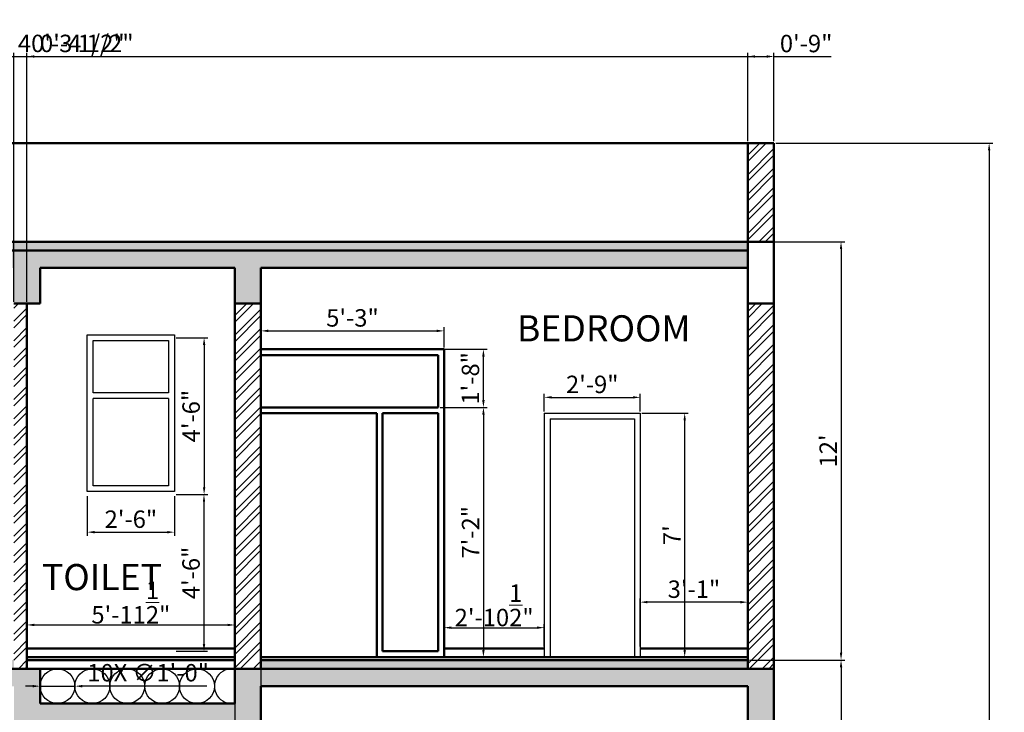
# Model space of a CAD drawing. Units: inches. Extents: x 1615 to 2231, y 1931 to 2519.
# Tile 6 of 6: x 1892 to 2231, y 2281 to 2519. Entities that reach past the tile are written whole.
import ezdxf

# ---------------------------------------------------------------- set-up
doc = ezdxf.new("R2010")
doc.units = ezdxf.units.IN
for name, color, linetype, lineweight in [('A-ANNO-DIMS', 2, 'Continuous', 18), ('A-AREA-IDEN', 7, 'Continuous', 25), ('A-DOOR', 3, 'Continuous', 25), ('A-GLAZ', 4, 'Continuous', 25), ('A-SECT', 7, 'Continuous', 50), ('A-WALL-PATT', 8, 'Continuous', 13), ('S-SLAB', 7, 'Continuous', 25)]:
    doc.layers.add(name, color=color, linetype=linetype, lineweight=lineweight)
doc.styles.get("Standard").update_dxf_attribs({"font": 'arial.ttf'})
doc.dimstyles.new('ISO-25', dxfattribs={"dimtxt": 6, "dimasz": 2.5, "dimexe": 1.25, "dimexo": 0.625, "dimtad": 1, "dimdec": 1, "dimlunit": 4, "dimtxsty": 'Standard', "dimcen": 2.5, "dimadec": 0, "dimazin": 0, "dimtfac": 1, "dimtdec": 1, "dimtmove": 0, "dimatfit": 3, "dimfxl": 1, "dimarcsym": 0})

# ---------------------------------------------------------------- blocks, each defined once
blk = doc.blocks.new('*D37')
at = {"layer": 'A-ANNO-DIMS', "color": 0, "lineweight": -2, "transparency": 16777216}
for p, q in [((1915.12, 2354.9), (1915.12, 2341.31)), ((1945.12, 2354.9), (1945.12, 2341.31)), ((1917.62, 2342.56), (1942.62, 2342.56))]:
    blk.add_line(p, q, dxfattribs=at)
at = {"layer": 'A-ANNO-DIMS', "color": 0, "lineweight": 100, "transparency": 16777216}
for points in [[(1917.62, 2342.98), (1917.62, 2342.14), (1915.12, 2342.56)], [(1942.62, 2342.98), (1942.62, 2342.14), (1945.12, 2342.56)]]:
    blk.add_solid(points, dxfattribs=at)
at = {"layer": 'Defpoints', "color": 0, "lineweight": 100, "transparency": 16777216}
for p in [(1915.12, 2355.53), (1945.12, 2355.53), (1945.12, 2342.56)]:
    blk.add_point(p, dxfattribs=at)
at = {"layer": 'A-ANNO-DIMS', "color": 0, "transparency": 16777216, "insert": (1930.12, 2346.25), "char_height": 6, "attachment_point": 5}
blk.add_mtext('2\'-6"', dxfattribs=at)
blk = doc.blocks.new('*D38')
at = {"layer": 'A-ANNO-DIMS', "color": 0, "lineweight": -2, "transparency": 16777216}
for p, q in [((1945.74, 2409.53), (1956.57, 2409.53)), ((1955.32, 2407.03), (1955.32, 2358.03)), ((1945.74, 2355.53), (1956.57, 2355.53))]:
    blk.add_line(p, q, dxfattribs=at)
at = {"layer": 'A-ANNO-DIMS', "color": 0, "lineweight": 100, "transparency": 16777216}
for points in [[(1954.91, 2407.03), (1955.74, 2407.03), (1955.32, 2409.53)], [(1954.91, 2358.03), (1955.74, 2358.03), (1955.32, 2355.53)]]:
    blk.add_solid(points, dxfattribs=at)
at = {"layer": 'Defpoints', "color": 0, "lineweight": 100, "transparency": 16777216}
for p in [(1945.12, 2409.53), (1945.12, 2355.53), (1955.32, 2355.53)]:
    blk.add_point(p, dxfattribs=at)
at = {"layer": 'A-ANNO-DIMS', "color": 0, "transparency": 16777216, "insert": (1951.63, 2382.53), "char_height": 6, "attachment_point": 5, "rotation": 90}
blk.add_mtext('4\'-6"', dxfattribs=at)
blk = doc.blocks.new('*D39')
at = {"layer": 'A-ANNO-DIMS', "color": 0, "lineweight": -2, "transparency": 16777216}
for p, q in [((1945.74, 2355.53), (1956.53, 2355.53)), ((1955.28, 2353.03), (1955.28, 2304.03)), ((1945.74, 2301.53), (1956.53, 2301.53))]:
    blk.add_line(p, q, dxfattribs=at)
at = {"layer": 'A-ANNO-DIMS', "color": 0, "lineweight": 100, "transparency": 16777216}
for points in [[(1954.87, 2353.03), (1955.7, 2353.03), (1955.28, 2355.53)], [(1954.87, 2304.03), (1955.7, 2304.03), (1955.28, 2301.53)]]:
    blk.add_solid(points, dxfattribs=at)
at = {"layer": 'Defpoints', "color": 0, "lineweight": 100, "transparency": 16777216}
for p in [(1945.12, 2355.53), (1945.12, 2301.53), (1955.28, 2301.53)]:
    blk.add_point(p, dxfattribs=at)
at = {"layer": 'A-ANNO-DIMS', "color": 0, "transparency": 16777216, "insert": (1951.6, 2328.53), "char_height": 6, "attachment_point": 5, "rotation": 90}
blk.add_mtext('4\'-6"', dxfattribs=at)
blk = doc.blocks.new('*D46')
at = {"layer": 'A-ANNO-DIMS', "color": 0, "lineweight": -2, "transparency": 16777216}
for p, q in [((2037.87, 2303.15), (2037.87, 2310.92)), ((2072.37, 2303.15), (2072.37, 2310.92)), ((2040.37, 2309.67), (2069.87, 2309.67))]:
    blk.add_line(p, q, dxfattribs=at)
at = {"layer": 'A-ANNO-DIMS', "color": 0, "lineweight": 100, "transparency": 16777216}
for points in [[(2040.37, 2310.09), (2040.37, 2309.25), (2037.87, 2309.67)], [(2069.87, 2310.09), (2069.87, 2309.25), (2072.37, 2309.67)]]:
    blk.add_solid(points, dxfattribs=at)
at = {"layer": 'Defpoints', "color": 0, "lineweight": 100, "transparency": 16777216}
for p in [(2072.37, 2309.67), (2037.87, 2302.53), (2072.37, 2302.53)]:
    blk.add_point(p, dxfattribs=at)
at = {"layer": 'A-ANNO-DIMS', "color": 0, "transparency": 16777216, "insert": (2055.12, 2317.37), "char_height": 6, "attachment_point": 5}
blk.add_mtext('2\'-10{\\H1x;\\S1/2;}"', dxfattribs=at)
blk = doc.blocks.new('*D47')
at = {"layer": 'A-ANNO-DIMS', "color": 0, "lineweight": -2, "transparency": 16777216}
for p, q in [((2105.99, 2383.53), (2121.93, 2383.53)), ((2120.68, 2302.03), (2120.68, 2381.03)), ((2105.99, 2299.53), (2121.93, 2299.53))]:
    blk.add_line(p, q, dxfattribs=at)
at = {"layer": 'A-ANNO-DIMS', "color": 0, "lineweight": 100, "transparency": 16777216}
for points in [[(2120.27, 2381.03), (2121.1, 2381.03), (2120.68, 2383.53)], [(2120.27, 2302.03), (2121.1, 2302.03), (2120.68, 2299.53)]]:
    blk.add_solid(points, dxfattribs=at)
at = {"layer": 'Defpoints', "color": 0, "lineweight": 100, "transparency": 16777216}
for p in [(2105.37, 2383.53), (2120.68, 2383.53), (2105.37, 2299.53)]:
    blk.add_point(p, dxfattribs=at)
at = {"layer": 'A-ANNO-DIMS', "color": 0, "transparency": 16777216, "insert": (2117.06, 2341.53), "char_height": 6, "attachment_point": 5, "rotation": 90}
blk.add_mtext("7'", dxfattribs=at)
blk = doc.blocks.new('*D48')
at = {"layer": 'A-ANNO-DIMS', "color": 0, "lineweight": -2, "transparency": 16777216}
for p, q in [((2072.37, 2384.15), (2072.37, 2390.23)), ((2074.87, 2388.98), (2102.87, 2388.98)), ((2105.37, 2384.15), (2105.37, 2390.23))]:
    blk.add_line(p, q, dxfattribs=at)
at = {"layer": 'A-ANNO-DIMS', "color": 0, "lineweight": 100, "transparency": 16777216}
for points in [[(2074.87, 2389.4), (2074.87, 2388.57), (2072.37, 2388.98)], [(2102.87, 2389.4), (2102.87, 2388.57), (2105.37, 2388.98)]]:
    blk.add_solid(points, dxfattribs=at)
at = {"layer": 'Defpoints', "color": 0, "lineweight": 100, "transparency": 16777216}
for p in [(2105.37, 2388.98), (2072.37, 2383.53), (2105.37, 2383.53)]:
    blk.add_point(p, dxfattribs=at)
at = {"layer": 'A-ANNO-DIMS', "color": 0, "transparency": 16777216, "insert": (2088.87, 2392.67), "char_height": 6, "attachment_point": 5}
blk.add_mtext('2\'-9"', dxfattribs=at)
blk = doc.blocks.new('*D54')
at = {"layer": 'A-ANNO-DIMS', "color": 0, "lineweight": -2, "transparency": 16777216}
for p, q in [((2036.49, 2405.53), (2052.68, 2405.53)), ((2051.43, 2388.03), (2051.43, 2403.03)), ((2036.49, 2385.53), (2052.68, 2385.53))]:
    blk.add_line(p, q, dxfattribs=at)
at = {"layer": 'A-ANNO-DIMS', "color": 0, "lineweight": 100, "transparency": 16777216}
for points in [[(2051.01, 2403.03), (2051.85, 2403.03), (2051.43, 2405.53)], [(2051.01, 2388.03), (2051.85, 2388.03), (2051.43, 2385.53)]]:
    blk.add_solid(points, dxfattribs=at)
at = {"layer": 'Defpoints', "color": 0, "lineweight": 100, "transparency": 16777216}
for p in [(2035.87, 2405.53), (2051.43, 2405.53), (2035.87, 2385.53)]:
    blk.add_point(p, dxfattribs=at)
at = {"layer": 'A-ANNO-DIMS', "color": 0, "transparency": 16777216, "insert": (2047.74, 2395.53), "char_height": 6, "attachment_point": 5, "rotation": 90}
blk.add_mtext('1\'-8"', dxfattribs=at)
blk = doc.blocks.new('*D55')
at = {"layer": 'A-ANNO-DIMS', "color": 0, "lineweight": -2, "transparency": 16777216}
for p, q in [((2036.49, 2385.53), (2052.68, 2385.53)), ((2051.43, 2383.03), (2051.43, 2302.03)), ((2036.49, 2299.53), (2052.68, 2299.53))]:
    blk.add_line(p, q, dxfattribs=at)
at = {"layer": 'A-ANNO-DIMS', "color": 0, "lineweight": 100, "transparency": 16777216}
for points in [[(2051.01, 2383.03), (2051.85, 2383.03), (2051.43, 2385.53)], [(2051.01, 2302.03), (2051.85, 2302.03), (2051.43, 2299.53)]]:
    blk.add_solid(points, dxfattribs=at)
at = {"layer": 'Defpoints', "color": 0, "lineweight": 100, "transparency": 16777216}
for p in [(2035.87, 2385.53), (2035.87, 2299.53), (2051.43, 2299.53)]:
    blk.add_point(p, dxfattribs=at)
at = {"layer": 'A-ANNO-DIMS', "color": 0, "transparency": 16777216, "insert": (2047.79, 2342.53), "char_height": 6, "attachment_point": 5, "rotation": 90}
blk.add_mtext('7\'-2"', dxfattribs=at)
blk = doc.blocks.new('*D56')
at = {"layer": 'A-ANNO-DIMS', "color": 0, "lineweight": -2, "transparency": 16777216}
for p, q in [((1974.87, 2406.15), (1974.87, 2413.12)), ((2037.87, 2406.15), (2037.87, 2413.12)), ((1977.37, 2411.87), (2035.37, 2411.87))]:
    blk.add_line(p, q, dxfattribs=at)
at = {"layer": 'A-ANNO-DIMS', "color": 0, "lineweight": 100, "transparency": 16777216}
for points in [[(1977.37, 2412.29), (1977.37, 2411.46), (1974.87, 2411.87)], [(2035.37, 2412.29), (2035.37, 2411.46), (2037.87, 2411.87)]]:
    blk.add_solid(points, dxfattribs=at)
at = {"layer": 'Defpoints', "color": 0, "lineweight": 100, "transparency": 16777216}
for p in [(2037.87, 2411.87), (1974.87, 2405.53), (2037.87, 2405.53)]:
    blk.add_point(p, dxfattribs=at)
at = {"layer": 'A-ANNO-DIMS', "color": 0, "transparency": 16777216, "insert": (2006.37, 2415.56), "char_height": 6, "attachment_point": 5}
blk.add_mtext('5\'-3"', dxfattribs=at)
blk = doc.blocks.new('*D57')
at = {"layer": 'A-ANNO-DIMS', "color": 0, "lineweight": -2, "transparency": 16777216}
for p, q in [((2105.37, 2303.15), (2105.37, 2319.71)), ((2139.87, 2318.46), (2107.87, 2318.46)), ((2142.37, 2303.15), (2142.37, 2319.71))]:
    blk.add_line(p, q, dxfattribs=at)
at = {"layer": 'A-ANNO-DIMS', "color": 0, "lineweight": 100, "transparency": 16777216}
for points in [[(2107.87, 2318.88), (2107.87, 2318.05), (2105.37, 2318.46)], [(2139.87, 2318.88), (2139.87, 2318.05), (2142.37, 2318.46)]]:
    blk.add_solid(points, dxfattribs=at)
at = {"layer": 'Defpoints', "color": 0, "lineweight": 100, "transparency": 16777216}
for p in [(2105.37, 2318.46), (2105.37, 2302.53), (2142.37, 2302.53)]:
    blk.add_point(p, dxfattribs=at)
at = {"layer": 'A-ANNO-DIMS', "color": 0, "transparency": 16777216, "insert": (2123.87, 2322.15), "char_height": 6, "attachment_point": 5}
blk.add_mtext('3\'-1"', dxfattribs=at)
blk = doc.blocks.new('*D61')
at = {"layer": 'A-ANNO-DIMS', "color": 0, "lineweight": -2, "transparency": 16777216}
for p, q in [((1894.37, 2303.15), (1894.37, 2311.86)), ((1896.87, 2310.61), (1963.37, 2310.61)), ((1965.87, 2303.15), (1965.87, 2311.86))]:
    blk.add_line(p, q, dxfattribs=at)
at = {"layer": 'A-ANNO-DIMS', "color": 0, "lineweight": 100, "transparency": 16777216}
for points in [[(1896.87, 2311.03), (1896.87, 2310.19), (1894.37, 2310.61)], [(1963.37, 2311.03), (1963.37, 2310.19), (1965.87, 2310.61)]]:
    blk.add_solid(points, dxfattribs=at)
at = {"layer": 'Defpoints', "color": 0, "lineweight": 100, "transparency": 16777216}
for p in [(1965.87, 2310.61), (1894.37, 2302.53), (1965.87, 2302.53)]:
    blk.add_point(p, dxfattribs=at)
at = {"layer": 'A-ANNO-DIMS', "color": 0, "transparency": 16777216, "insert": (1930.12, 2318.31), "char_height": 6, "attachment_point": 5}
blk.add_mtext('5\'-11{\\H1x;\\S1/2;}"', dxfattribs=at)
blk = doc.blocks.new('*D62')
at = {"layer": 'A-ANNO-DIMS', "color": 0, "lineweight": -2, "transparency": 16777216}
for p, q in [((2142.99, 2442.53), (2175.73, 2442.53)), ((2174.48, 2440.03), (2174.48, 2301.03)), ((2142.99, 2298.53), (2175.73, 2298.53))]:
    blk.add_line(p, q, dxfattribs=at)
at = {"layer": 'A-ANNO-DIMS', "color": 0, "lineweight": 100, "transparency": 16777216}
for points in [[(2174.07, 2440.03), (2174.9, 2440.03), (2174.48, 2442.53)], [(2174.07, 2301.03), (2174.9, 2301.03), (2174.48, 2298.53)]]:
    blk.add_solid(points, dxfattribs=at)
at = {"layer": 'Defpoints', "color": 0, "lineweight": 100, "transparency": 16777216}
for p in [(2142.37, 2442.53), (2142.37, 2298.53), (2174.48, 2298.53)]:
    blk.add_point(p, dxfattribs=at)
at = {"layer": 'A-ANNO-DIMS', "color": 0, "transparency": 16777216, "insert": (2170.85, 2370.53), "char_height": 6, "attachment_point": 5, "rotation": 90}
blk.add_mtext("12'", dxfattribs=at)
blk = doc.blocks.new('*D63')
at = {"layer": 'A-ANNO-DIMS', "color": 0, "lineweight": -2, "transparency": 16777216}
for p, q in [((2142.99, 2298.53), (2175.73, 2298.53)), ((2174.48, 2296.03), (2174.48, 2157.03)), ((2142.99, 2154.53), (2175.73, 2154.53))]:
    blk.add_line(p, q, dxfattribs=at)
at = {"layer": 'A-ANNO-DIMS', "color": 0, "lineweight": 100, "transparency": 16777216}
for points in [[(2174.07, 2296.03), (2174.9, 2296.03), (2174.48, 2298.53)], [(2174.07, 2157.03), (2174.9, 2157.03), (2174.48, 2154.53)]]:
    blk.add_solid(points, dxfattribs=at)
at = {"layer": 'Defpoints', "color": 0, "lineweight": 100, "transparency": 16777216}
for p in [(2142.37, 2298.53), (2142.37, 2154.53), (2174.48, 2154.53)]:
    blk.add_point(p, dxfattribs=at)
at = {"layer": 'A-ANNO-DIMS', "color": 0, "transparency": 16777216, "insert": (2170.85, 2226.53), "char_height": 6, "attachment_point": 5, "rotation": 90}
blk.add_mtext("12'", dxfattribs=at)
blk = doc.blocks.new('WIN-TOILET')
for p, q in [((1915.12, 2410.53), (1945.12, 2410.53)), ((1915.12, 2356.53), (1915.12, 2410.53)), ((1945.12, 2410.53), (1945.12, 2390.53)), ((1917.12, 2408.53), (1943.12, 2408.53)), ((1917.12, 2390.53), (1917.12, 2408.53)), ((1943.12, 2408.53), (1943.12, 2390.53)), ((1943.12, 2390.53), (1917.12, 2390.53)), ((1943.12, 2388.53), (1917.12, 2388.53)), ((1917.12, 2358.53), (1917.12, 2388.53)), ((1943.12, 2388.53), (1943.12, 2358.53)), ((1945.12, 2390.53), (1945.12, 2356.53)), ((1943.12, 2358.53), (1917.12, 2358.53)), ((1945.12, 2356.53), (1915.12, 2356.53))]:
    blk.add_line(p, q)
blk = doc.blocks.new('DOOR-KITCHEN')
for p, q in [((2072.37, 2383.53), (2072.37, 2299.53)), ((2072.37, 2383.53), (2105.37, 2383.53)), ((2105.37, 2383.53), (2105.37, 2299.53)), ((2074.37, 2381.53), (2103.37, 2381.53)), ((2074.37, 2381.53), (2074.37, 2299.53)), ((2103.37, 2381.53), (2103.37, 2299.53))]:
    blk.add_line(p, q)
blk = doc.blocks.new('*D78')
at = {"layer": 'A-ANNO-DIMS', "color": 0, "lineweight": -2, "transparency": 16777216}
for p, q in [((1667.87, 2477.15), (1667.87, 2507.6)), ((2151.37, 2477.15), (2151.37, 2507.6)), ((1670.37, 2506.35), (2148.87, 2506.35))]:
    blk.add_line(p, q, dxfattribs=at)
at = {"layer": 'A-ANNO-DIMS', "color": 0, "lineweight": 100, "transparency": 16777216}
for points in [[(1670.37, 2506.77), (1670.37, 2505.93), (1667.87, 2506.35)], [(2148.87, 2506.77), (2148.87, 2505.93), (2151.37, 2506.35)]]:
    blk.add_solid(points, dxfattribs=at)
at = {"layer": 'Defpoints', "color": 0, "lineweight": 100, "transparency": 16777216}
for p in [(2151.37, 2506.35), (1667.87, 2476.53), (2151.37, 2476.53)]:
    blk.add_point(p, dxfattribs=at)
at = {"layer": 'A-ANNO-DIMS', "color": 0, "transparency": 16777216, "insert": (1909.62, 2510.08), "char_height": 6, "attachment_point": 5}
blk.add_mtext('40\'-3 1/2"', dxfattribs=at)
blk = doc.blocks.new('*D79')
at = {"layer": 'A-ANNO-DIMS', "color": 0, "lineweight": -2, "transparency": 16777216}
for p, q in [((2151.99, 2476.53), (2226.69, 2476.53)), ((2225.44, 2474.03), (2225.44, 2004.53)), ((2175.99, 2002.03), (2226.69, 2002.03))]:
    blk.add_line(p, q, dxfattribs=at)
at = {"layer": 'A-ANNO-DIMS', "color": 0, "lineweight": 100, "transparency": 16777216}
for points in [[(2225.02, 2474.03), (2225.86, 2474.03), (2225.44, 2476.53)], [(2225.02, 2004.53), (2225.86, 2004.53), (2225.44, 2002.03)]]:
    blk.add_solid(points, dxfattribs=at)
at = {"layer": 'Defpoints', "color": 0, "lineweight": 100, "transparency": 16777216}
for p in [(2151.37, 2476.53), (2175.37, 2002.03), (2225.44, 2002.03)]:
    blk.add_point(p, dxfattribs=at)
at = {"layer": 'A-ANNO-DIMS', "color": 0, "transparency": 16777216, "insert": (2221.71, 2239.28), "char_height": 6, "attachment_point": 5, "rotation": 90}
blk.add_mtext('39\'-6 1/2"', dxfattribs=at)
blk = doc.blocks.new('*D81')
at = {"layer": 'A-ANNO-DIMS', "color": 0, "lineweight": -2, "transparency": 16777216}
for p, q in [((2142.37, 2477.15), (2142.37, 2507.6)), ((2151.37, 2477.15), (2151.37, 2507.6)), ((2144.87, 2506.35), (2148.87, 2506.35)), ((2151.37, 2506.35), (2171.07, 2506.35))]:
    blk.add_line(p, q, dxfattribs=at)
at = {"layer": 'A-ANNO-DIMS', "color": 0, "lineweight": 100, "transparency": 16777216}
for points in [[(2144.87, 2506.77), (2144.87, 2505.93), (2142.37, 2506.35)], [(2148.87, 2506.77), (2148.87, 2505.93), (2151.37, 2506.35)]]:
    blk.add_solid(points, dxfattribs=at)
at = {"layer": 'Defpoints', "color": 0, "lineweight": 100, "transparency": 16777216}
for p in [(2151.37, 2506.35), (2142.37, 2476.53), (2151.37, 2476.53)]:
    blk.add_point(p, dxfattribs=at)
at = {"layer": 'A-ANNO-DIMS', "color": 0, "transparency": 16777216, "insert": (2162.47, 2510.04), "char_height": 6, "attachment_point": 5}
blk.add_mtext('0\'-9"', dxfattribs=at)
blk = doc.blocks.new('*D82')
at = {"layer": 'A-ANNO-DIMS', "color": 0, "lineweight": -2, "transparency": 16777216}
for p, q in [((1889.87, 2421.92), (1889.87, 2507.6)), ((1894.37, 2421.92), (1894.37, 2507.6)), ((1887.37, 2506.35), (1884.87, 2506.35)), ((1889.87, 2506.35), (1894.37, 2506.35)), ((1896.87, 2506.35), (1930.55, 2506.35))]:
    blk.add_line(p, q, dxfattribs=at)
at = {"layer": 'A-ANNO-DIMS', "color": 0, "lineweight": 100, "transparency": 16777216}
for points in [[(1887.37, 2506.77), (1887.37, 2505.93), (1889.87, 2506.35)], [(1896.87, 2506.77), (1896.87, 2505.93), (1894.37, 2506.35)]]:
    blk.add_solid(points, dxfattribs=at)
at = {"layer": 'Defpoints', "color": 0, "lineweight": 100, "transparency": 16777216}
for p in [(1894.37, 2506.35), (1889.87, 2421.29), (1894.37, 2421.29)]:
    blk.add_point(p, dxfattribs=at)
at = {"layer": 'A-ANNO-DIMS', "color": 0, "transparency": 16777216, "insert": (1914.96, 2510.08), "char_height": 6, "attachment_point": 5}
blk.add_mtext('0\'-4 1/2"', dxfattribs=at)
blk = doc.blocks.new('*D83')
at = {"layer": 'A-ANNO-DIMS', "color": 0, "lineweight": -2, "transparency": 16777216}
for p, q in [((1965.87, 2420.67), (1965.87, 1970.95)), ((1974.87, 2420.67), (1974.87, 1970.95)), ((1968.37, 1972.2), (1972.37, 1972.2)), ((1974.87, 1972.2), (1994.57, 1972.2))]:
    blk.add_line(p, q, dxfattribs=at)
at = {"layer": 'A-ANNO-DIMS', "color": 0, "lineweight": 100, "transparency": 16777216}
for points in [[(1968.37, 1972.62), (1968.37, 1971.78), (1965.87, 1972.2)], [(1972.37, 1972.62), (1972.37, 1971.78), (1974.87, 1972.2)]]:
    blk.add_solid(points, dxfattribs=at)
at = {"layer": 'Defpoints', "color": 0, "lineweight": 100, "transparency": 16777216}
for p in [(1965.87, 2421.29), (1974.87, 2421.29), (1974.87, 1972.2)]:
    blk.add_point(p, dxfattribs=at)
at = {"layer": 'A-ANNO-DIMS', "color": 0, "transparency": 16777216, "insert": (1985.97, 1975.89), "char_height": 6, "attachment_point": 5}
blk.add_mtext('0\'-9"', dxfattribs=at)
blk = doc.blocks.new('*D91')
at = {"layer": 'A-ANNO-DIMS', "color": 0, "lineweight": -2, "transparency": 16777216}
for p, q in [((1896.37, 2289.53), (1893.87, 2289.53)), ((1898.87, 2289.53), (1910.87, 2289.53)), ((1956.26, 2289.53), (1913.37, 2289.53))]:
    blk.add_line(p, q, dxfattribs=at)
at = {"layer": 'A-ANNO-DIMS', "color": 0, "lineweight": 100, "transparency": 16777216}
for points in [[(1896.37, 2289.94), (1896.37, 2289.11), (1898.87, 2289.53)], [(1913.37, 2289.94), (1913.37, 2289.11), (1910.87, 2289.53)]]:
    blk.add_solid(points, dxfattribs=at)
at = {"layer": 'Defpoints', "color": 0, "lineweight": 100, "transparency": 16777216}
for p in [(1898.87, 2289.53), (1910.87, 2289.53)]:
    blk.add_point(p, dxfattribs=at)
at = {"layer": 'A-ANNO-DIMS', "color": 0, "transparency": 16777216, "insert": (1936.06, 2293.38), "char_height": 6, "attachment_point": 5, "rotation": 0.0032}
blk.add_mtext('10X ∅1\'-0"', dxfattribs=at)

msp = doc.modelspace()

# ---------------------------------------------------------------- hatches: boundary and pattern name
at = {"layer": 'A-WALL-PATT'}
h = msp.add_hatch(dxfattribs=at)
h.set_pattern_fill('ANSI32', color=256, scale=0.5)
h.paths.add_polyline_path([(1676.87, 2421.53), (1667.87, 2421.53), (1667.87, 2295.53), (1676.87, 2295.53)])
h.paths.add_polyline_path([(1676.87, 2277.53), (1667.87, 2277.53), (1667.87, 2151.53), (1676.87, 2151.53)])
h.paths.add_polyline_path([(1676.87, 2476.53), (1667.87, 2476.53), (1667.87, 2439.53), (1676.87, 2439.53)])
h.paths.add_polyline_path([(1894.37, 2421.29), (1889.87, 2421.29), (1889.87, 2295.53), (1894.37, 2295.53)])
h.paths.add_polyline_path([(1974.87, 2421.29), (1965.87, 2421.29), (1965.87, 2295.53), (1974.87, 2295.53)])
h.paths.add_polyline_path([(2151.37, 2421.29), (2142.37, 2421.29), (2142.37, 2295.53), (2151.37, 2295.53)])
h.paths.add_polyline_path([(2151.37, 2476.53), (2142.37, 2476.53), (2142.37, 2442.53), (2151.37, 2442.53)])
h.paths.add_polyline_path([(1974.87, 2277.53), (1965.87, 2277.53), (1965.87, 2151.53), (1974.87, 2151.53)])
h.paths.add_polyline_path([(1974.87, 2133.53), (1965.87, 2133.53), (1965.87, 2060.03), (1974.87, 2060.03)])
h.paths.add_polyline_path([(2098.87, 2145.53), (2094.37, 2145.53), (2094.37, 2059.03), (2098.87, 2059.03)])
h = msp.add_hatch(dxfattribs=at)
h.set_pattern_fill('AR-CONC', color=256, scale=0.1)
h.paths.add_polyline_path([(1898.87, 2151.53), (1667.87, 2151.53), (1667.87, 2145.53), (1679.87, 2145.53), (1682.87, 2145.53), (1889.87, 2145.53), (1889.87, 2133.53), (1974.87, 2133.53), (1974.87, 2145.53), (2142.37, 2145.53), (2142.37, 2133.53), (2157.37, 2133.53), (2157.37, 2151.53), (2155.87, 2151.53), (2151.37, 2151.53), (1965.87, 2151.53), (1965.87, 2139.53), (1898.87, 2139.53)])
h.paths.add_polyline_path([(1898.87, 2295.53), (1667.87, 2295.53), (1667.87, 2277.53), (1676.87, 2277.53), (1676.87, 2289.53), (1889.87, 2289.53), (1889.87, 2277.53), (1974.87, 2277.53), (1974.87, 2289.53), (2142.37, 2289.53), (2142.37, 2277.53), (2151.37, 2277.53), (2151.37, 2295.53), (1965.87, 2295.53), (1965.87, 2283.53), (1898.87, 2283.53)])
h.paths.add_polyline_path([(2142.37, 2439.53), (1676.87, 2439.53), (1667.87, 2439.53), (1667.87, 2421.53), (1676.87, 2421.53), (1676.87, 2433.53), (1889.87, 2433.53), (1889.87, 2421.29), (1898.87, 2421.29), (1898.87, 2433.53), (1965.87, 2433.53), (1965.87, 2421.29), (1974.87, 2421.29), (1974.87, 2433.53), (2142.37, 2433.53)])
h = msp.add_hatch(dxfattribs=at)
h.set_pattern_fill('DOTS', color=256, scale=0.5)
h.paths.add_polyline_path([(2142.37, 2442.53), (1839.37, 2442.53), (1676.87, 2442.53), (1676.87, 2439.53), (2142.37, 2439.53)])
h.paths.add_polyline_path([(1889.87, 2298.53), (1676.87, 2298.53), (1676.87, 2295.53), (1889.87, 2295.53)])
h.paths.add_polyline_path([(2142.37, 2298.53), (1974.87, 2298.53), (1974.87, 2295.53), (2142.37, 2295.53)])
h.paths.add_polyline_path([(1889.87, 2154.53), (1676.87, 2154.53), (1676.87, 2151.53), (1889.87, 2151.53)])
h.paths.add_polyline_path([(1965.87, 2154.53), (1894.37, 2154.53), (1894.37, 2151.53), (1965.87, 2151.53)])
h.paths.add_polyline_path([(2142.37, 2154.53), (1974.87, 2154.53), (1974.87, 2151.53), (2142.37, 2151.53)])
h.paths.add_polyline_path([(2094.37, 2062.03), (1974.87, 2062.03), (1974.87, 2059.03), (2094.37, 2059.03)])
h.paths.add_polyline_path([(2142.37, 2062.03), (2098.87, 2062.03), (2098.87, 2059.03), (2142.37, 2059.03)])
h.paths.add_polyline_path([(1956.87, 2049.53), (1693.37, 2049.53), (1693.37, 2046.53), (1956.87, 2046.53)])

# ---------------------------------------------------------------- linework, layer by layer
at = {"layer": 'A-SECT'}
for p, q in [((1667.87, 2476.53), (2151.37, 2476.53)), ((2142.37, 2476.53), (2142.37, 2295.53)), ((2151.37, 2476.53), (2151.37, 2151.53)), ((1676.87, 2439.53), (2142.37, 2439.53)), ((1839.37, 2442.53), (2151.37, 2442.53)), ((1898.87, 2421.29), (1898.87, 2433.53)), ((1898.87, 2433.53), (1965.87, 2433.53)), ((1965.87, 2433.53), (1965.87, 2295.53)), ((1974.87, 2433.53), (1974.87, 2295.53)), ((1974.87, 2433.53), (2142.37, 2433.53)), ((1889.87, 2421.29), (1898.87, 2421.29)), ((1894.37, 2421.29), (1894.37, 2295.53)), ((1965.87, 2421.29), (1974.87, 2421.29)), ((2142.37, 2421.29), (2151.37, 2421.29)), ((1974.87, 2405.53), (2037.87, 2405.53)), ((2037.87, 2405.53), (2037.87, 2299.53)), ((1974.87, 2403.53), (2035.87, 2403.53)), ((2035.87, 2403.53), (2035.87, 2385.53)), ((1974.87, 2385.53), (2035.87, 2385.53)), ((1974.87, 2383.53), (2014.71, 2383.53)), ((2014.71, 2383.53), (2014.71, 2299.53)), ((2016.71, 2383.53), (2035.87, 2383.53)), ((2016.71, 2383.53), (2016.71, 2301.53)), ((2035.87, 2383.53), (2035.87, 2301.53)), ((1894.37, 2302.53), (1965.87, 2302.53)), ((2016.71, 2301.53), (2035.87, 2301.53)), ((2037.87, 2302.53), (2072.37, 2302.53)), ((2105.37, 2302.53), (2142.37, 2302.53)), ((1894.37, 2299.53), (1965.87, 2299.53)), ((1894.37, 2298.53), (1965.87, 2298.53)), ((1965.87, 2298.53), (1965.87, 2283.53)), ((1974.87, 2299.53), (2142.37, 2299.53)), ((1974.87, 2298.53), (2142.37, 2298.53)), ((1667.87, 2295.53), (2151.37, 2295.53)), ((1898.87, 2295.53), (1898.87, 2283.53)), ((1974.87, 2289.53), (1974.87, 2151.53)), ((1974.87, 2289.53), (2142.37, 2289.53)), ((2142.37, 2289.53), (2142.37, 2151.53)), ((1898.87, 2283.53), (1965.87, 2283.53))]:
    msp.add_line(p, q, dxfattribs=at)
at = {"layer": 'S-SLAB'}
for centre in [(1904.87, 2289.53), (1916.87, 2289.53), (1928.87, 2289.53), (1940.87, 2289.53), (1952.87, 2289.53)]:
    msp.add_circle(centre, 6, dxfattribs=at)
msp.add_arc((1964.87, 2289.53), 6, 80.4059, 279.5941, dxfattribs=at)

# ---------------------------------------------------------------- block references
at = {"layer": 'A-DOOR'}
msp.add_blockref('DOOR-KITCHEN', (0, 0), dxfattribs=at)
at = {"layer": 'A-GLAZ'}
msp.add_blockref('WIN-TOILET', (0, 0), dxfattribs=at)

# ---------------------------------------------------------------- texts
at = {"layer": 'A-AREA-IDEN', "char_height": 9, "attachment_point": 1}
for s, width, insert in [('BEDROOM', 2.6039, (2062.95, 2417.24)), ('TOILET', 1.0394, (1899.51, 2331.59))]:
    msp.add_mtext_dynamic_manual_height_columns(s, width=width, gutter_width=12.5, heights=[0], dxfattribs=dict(at, insert=insert))

# ---------------------------------------------------------------- dimensions: what is measured, and where the dimension line sits
at = {"layer": 'A-ANNO-DIMS'}
for base, p1, p2, override, picture, middle in [((2151.37, 2506.35), (1667.87, 2476.53), (2151.37, 2476.53), {"dimdec": 1, "dimlfac": 1, "dimrnd": 0, "dimzin": 1, "dimdsep": 46, "dimlunit": 4, "dimfrac": 2}, '*D78', (1909.62, 2510.08)), ((1894.37, 2506.35), (1889.87, 2421.29), (1894.37, 2421.29), {"dimdec": 1, "dimlfac": 1, "dimrnd": 0, "dimzin": 1, "dimdsep": 46, "dimlunit": 4, "dimfrac": 2}, '*D82', (1914.96, 2510.08)), ((2151.37, 2506.35), (2142.37, 2476.53), (2151.37, 2476.53), {"dimdec": 1, "dimlfac": 1, "dimrnd": 0, "dimzin": 1, "dimdsep": 46, "dimlunit": 4, "dimfrac": 2}, '*D81', (2162.47, 2510.04)), ((1974.87, 1972.2), (1965.87, 2421.29), (1974.87, 2421.29), {"dimdec": 1, "dimlfac": 1, "dimrnd": 0, "dimzin": 1, "dimdsep": 46, "dimlunit": 4, "dimfrac": 2}, '*D83', (1985.97, 1975.89)), ((2037.87, 2411.87), (1974.87, 2405.53), (2037.87, 2405.53), {"dimclrd": 0, "dimclre": 0, "dimclrt": 0}, '*D56', (2006.37, 2415.56)), ((2105.37, 2388.98), (2072.37, 2383.53), (2105.37, 2383.53), {"dimclrd": 0, "dimclre": 0, "dimclrt": 0}, '*D48', (2088.87, 2392.67)), ((1945.12, 2342.56), (1915.12, 2355.53), (1945.12, 2355.53), {"dimclrd": 0, "dimclre": 0, "dimclrt": 0}, '*D37', (1930.12, 2346.25)), ((1965.87, 2310.61), (1894.37, 2302.53), (1965.87, 2302.53), {"dimclrd": 0, "dimclre": 0, "dimclrt": 0}, '*D61', (1930.12, 2318.31)), ((2072.37, 2309.67), (2037.87, 2302.53), (2072.37, 2302.53), {"dimclrd": 0, "dimclre": 0, "dimclrt": 0}, '*D46', (2055.12, 2317.37)), ((2105.37, 2318.46), (2142.37, 2302.53), (2105.37, 2302.53), {"dimclrd": 0, "dimclre": 0, "dimclrt": 0}, '*D57', (2123.87, 2322.15))]:
    dim = msp.add_linear_dim(base=base, p1=p1, p2=p2, dimstyle='ISO-25', override=override, dxfattribs=at)
    dim.commit()
    dim.dimension.update_dxf_attribs({"geometry": picture, "text_midpoint": middle})
for base, p1, p2, override, picture, middle in [((2225.44, 2002.03), (2151.37, 2476.53), (2175.37, 2002.03), {"dimdec": 1, "dimlfac": 1, "dimrnd": 0, "dimzin": 1, "dimdsep": 46, "dimlunit": 4, "dimfrac": 2}, '*D79', (2221.71, 2239.28)), ((2174.48, 2298.53), (2142.37, 2442.53), (2142.37, 2298.53), {"dimclrd": 0, "dimclre": 0, "dimclrt": 0}, '*D62', (2170.85, 2370.53)), ((1955.32, 2355.53), (1945.12, 2409.53), (1945.12, 2355.53), {"dimclrd": 0, "dimclre": 0, "dimclrt": 0}, '*D38', (1951.63, 2382.53)), ((2051.43, 2405.53), (2035.87, 2385.53), (2035.87, 2405.53), {"dimclrd": 0, "dimclre": 0, "dimclrt": 0}, '*D54', (2047.74, 2395.53)), ((2051.43, 2299.53), (2035.87, 2385.53), (2035.87, 2299.53), {"dimclrd": 0, "dimclre": 0, "dimclrt": 0}, '*D55', (2047.79, 2342.53)), ((2120.68, 2383.53), (2105.37, 2299.53), (2105.37, 2383.53), {"dimclrd": 0, "dimclre": 0, "dimclrt": 0}, '*D47', (2117.06, 2341.53)), ((1955.28, 2301.53), (1945.12, 2355.53), (1945.12, 2301.53), {"dimclrd": 0, "dimclre": 0, "dimclrt": 0}, '*D39', (1951.6, 2328.53)), ((2174.48, 2154.53), (2142.37, 2298.53), (2142.37, 2154.53), {"dimclrd": 0, "dimclre": 0, "dimclrt": 0}, '*D63', (2170.85, 2226.53))]:
    dim = msp.add_linear_dim(base=base, p1=p1, p2=p2, angle=90, dimstyle='ISO-25', override=override, dxfattribs=at)
    dim.commit()
    dim.dimension.update_dxf_attribs({"geometry": picture, "text_midpoint": middle})
dim = msp.add_diameter_dim_2p(p1=(1898.87, 2289.53), p2=(1910.87, 2289.53), text='10X <>', dimstyle='ISO-25', override={"dimdec": 1, "dimlfac": 1, "dimrnd": 0, "dimzin": 1, "dimdsep": 46, "dimlunit": 4, "dimfrac": 2}, dxfattribs=at)
dim.commit()
dim.dimension.update_dxf_attribs({"geometry": '*D91', "text_midpoint": (1936.06, 2289.53)})

doc.saveas('drawing.dxf')
